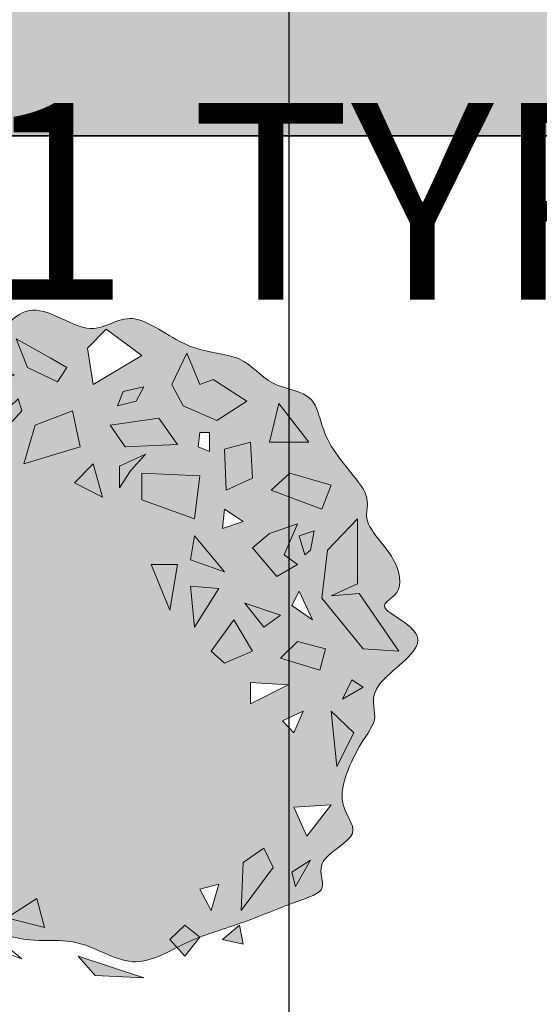
# Model space of a CAD drawing. Units: metres. Extents: x 4298.5 to 4325.2, y 2075 to 2095.8.
# Tile 9 of 35: x 4307.1445 to 4307.6197, y 2079.0337 to 2079.9341. Entities that reach past the tile are written whole.
import ezdxf

# ---------------------------------------------------------------- set-up
doc = ezdxf.new("R2010")
doc.units = ezdxf.units.M
for name, color, linetype, lineweight in [('A-ANNO-DIMS', 2, 'Continuous', 18), ('A-WALL', 7, 'Continuous', 35), ('A-WALL-PATT', 252, 'Continuous', 13), ('L-PLNT', 94, 'Continuous', 13)]:
    doc.layers.add(name, color=color, linetype=linetype, lineweight=lineweight)
doc.layers.add('L-PLNT-PATT', color=116, linetype='Continuous', lineweight=13, true_color=0x13823e)
doc.styles.get("Standard").update_dxf_attribs({"font": 'arial.ttf'})
doc.dimstyles.get("Standard").update_dxf_attribs({"dimtxt": 0.18, "dimasz": 0.18, "dimexe": 0.18, "dimexo": 0.0625, "dimgap": 0.09, "dimtad": 0, "dimtih": 1, "dimtoh": 1, "dimdec": 4, "dimzin": 0, "dimdsep": 46, "dimtxsty": 'Standard', "dimcen": 0.09, "dimadec": 0, "dimazin": 0, "dimtfac": 1, "dimtdec": 4, "dimtofl": 0, "dimtmove": 0, "dimatfit": 3, "dimfxl": 1, "dimtolj": 1, "dimtzin": 0, "dimarcsym": 0})

# ---------------------------------------------------------------- blocks, each defined once
blk = doc.blocks.new('*U9')
for points in [[(1.237, 12.003), (0.562, 11.31), (0.764, 10.013), (2.519, 11.051)], [(-2.003, 11.656), (-1.598, 10.618), (-0.518, 10.099), (-0.181, 10.618), (-0.788, 10.964)], [(-4.432, 11.051), (-5.175, 10.359), (-3.96, 9.493), (-2.07, 10.359)], [(4.139, 11.137), (3.599, 10.013), (4.004, 9.234), (5.218, 8.715), (6.298, 9.407), (5.083, 10.186), (4.611, 10.013)], [(-5.782, 9.753), (-7.537, 9.234), (-8.009, 7.504), (-6.255, 8.455)], [(2.586, 9.926), (1.844, 9.753), (1.642, 9.234), (2.316, 9.407)], [(-1.935, 9.493), (-2.475, 8.974), (-2.273, 8.542), (-1.8, 9.061)], [(7.446, 9.32), (7.108, 7.936), (8.525, 7.936)], [(-4.837, 8.628), (-3.825, 7.85), (-4.027, 8.974)], [(0.022, 9.061), (-1.328, 8.542), (-1.733, 7.157), (0.292, 7.763)], [(1.372, 8.542), (3.126, 8.801), (3.801, 7.85), (1.912, 7.763)], [(4.611, 8.282), (4.544, 7.763), (4.949, 7.59), (4.949, 8.282)], [(6.433, 7.936), (5.488, 7.676), (5.556, 6.206), (6.501, 6.638)], [(-2.88, 7.504), (-3.15, 6.638), (-2.273, 6.725)], [(1.709, 6.292), (1.709, 7.071), (2.654, 7.504), (2.114, 6.898)], [(0.764, 7.157), (0.089, 6.465), (1.102, 5.946)], [(-5.782, 6.811), (-6.659, 6.206), (-6.524, 5.687)], [(2.519, 6.811), (2.519, 5.86), (4.409, 5.167), (4.611, 6.725)], [(7.851, 6.811), (7.176, 6.206), (8.998, 5.514), (9.335, 6.379)], [(-8.144, 6.033), (-9.359, 5.946), (-9.022, 4.735)], [(-4.567, 6.379), (-5.445, 4.475), (-3.892, 4.821)], [(5.488, 5.514), (5.421, 4.821), (6.163, 5.081)], [(8.12, 4.994), (7.108, 4.648), (6.501, 4.129), (7.378, 3.091), (8.12, 3.524), (7.648, 3.87)], [(10.28, 5.167), (9.2, 4.043), (8.998, 2.312), (10.482, 0.495), (11.765, 0.409), (10.348, 2.485), (9.335, 2.399), (10.28, 2.831)], [(8.728, 4.735), (8.188, 4.562), (8.39, 3.87), (8.593, 4.043)], [(4.409, 4.562), (4.274, 3.697), (5.488, 3.264)], [(-11.316, 1.793), (-9.831, 2.312), (-9.629, 3.437), (-10.439, 3.524)], [(3.531, 1.88), (2.856, 3.524), (3.801, 3.524)], [(-8.212, 3.091), (-8.482, 2.312), (-7.874, 2.572)], [(4.274, 2.745), (5.286, 2.658), (4.409, 1.274)], [(8.188, 2.572), (7.918, 2.053), (8.66, 1.534)], [(7.513, 1.707), (6.906, 1.274), (6.231, 2.139)], [(-6.997, 1.793), (-7.942, 1.534), (-7.469, 0.495)], [(5.826, 1.534), (5.016, 0.409), (5.488, -0.024), (6.501, 0.409)], [(-8.212, 0.409), (-9.426, 0.322), (-9.831, 0.841)], [(8.12, 0.755), (7.513, 0.149), (8.93, -0.283), (9.133, 0.495)], [(10.078, -0.629), (9.74, -1.322), (10.482, -0.889)], [(7.783, -0.803), (6.433, -1.495), (6.433, -0.716)], [(8.323, -1.754), (7.985, -2.533), (7.581, -2.1)], [(9.335, -1.754), (9.538, -3.744), (10.145, -2.533)], [(-10.034, -2.706), (-10.641, -3.312), (-10.439, -4.436), (-9.899, -3.485)], [(-8.279, -5.734), (-6.794, -5.302), (-6.997, -6.513)], [(9.335, -5.129), (8.458, -6.253), (7.985, -5.215)], [(6.096, -8.935), (6.163, -7.205), (6.906, -6.686), (7.243, -7.378)], [(8.053, -8.07), (8.593, -7.118), (7.918, -7.551)], [(5.286, -7.984), (4.611, -8.157), (5.016, -8.935)], [(-2.34, -9.195), (-1.26, -8.503), (-0.99, -9.541)], [(-4.837, -8.849), (-4.432, -9.454), (-5.985, -9.801)], [(4.071, -9.454), (3.531, -9.974), (4.071, -10.579), (4.611, -9.887)], [(6.028, -9.454), (5.421, -9.974), (6.163, -10.147)], [(-2.543, -10.06), (-3.015, -10.233), (-1.8, -10.666)], [(0.224, -10.579), (0.832, -11.272), (2.586, -11.358)]]:
    blk.add_lwpolyline(points, close=True)
blk = doc.blocks.new('*D23')
at = {"layer": 'A-ANNO-DIMS', "color": 0, "lineweight": -2, "transparency": 16777216}
for p, q in [((4308.16058, 2079.85556), (4308.16058, 2079.58806)), ((4309.16058, 2079.85556), (4309.16058, 2079.58806)), ((4308.16058, 2079.76806), (4307.98058, 2079.76806)), ((4308.98058, 2079.76806), (4308.34058, 2079.76806))]:
    blk.add_line(p, q, dxfattribs=at)
at = {"layer": 'A-ANNO-DIMS', "color": 0, "transparency": 16777216}
for points in [[(4308.34058, 2079.79806), (4308.34058, 2079.73806), (4308.16058, 2079.76806)], [(4308.98058, 2079.79806), (4308.98058, 2079.73806), (4309.16058, 2079.76806)]]:
    blk.add_solid(points, dxfattribs=at)
at = {"layer": 'Defpoints', "color": 0, "transparency": 16777216}
for p in [(4308.16058, 2079.91806), (4309.16058, 2079.91806), (4308.16058, 2079.76806)]:
    blk.add_point(p, dxfattribs=at)
at = {"layer": 'A-ANNO-DIMS', "color": 0, "transparency": 16777216, "insert": (4306.70861, 2079.76806), "char_height": 0.18, "attachment_point": 5}
blk.add_mtext('\\A1;WINDOW W1 1 TYP.', dxfattribs=at)
blk = doc.blocks.new('*D47')
at = {"layer": 'A-ANNO-DIMS', "color": 0, "lineweight": -2, "transparency": 16777216}
for p, q in [((4300.43058, 2084.49556), (4300.43058, 2074.98956)), ((4322.81058, 2084.49556), (4322.81058, 2074.98956)), ((4300.61058, 2075.16956), (4311.22515, 2075.16956)), ((4322.63058, 2075.16956), (4312.016, 2075.16956))]:
    blk.add_line(p, q, dxfattribs=at)
at = {"layer": 'A-ANNO-DIMS', "color": 0, "transparency": 16777216}
for points in [[(4300.61058, 2075.19956), (4300.61058, 2075.13956), (4300.43058, 2075.16956)], [(4322.63058, 2075.19956), (4322.63058, 2075.13956), (4322.81058, 2075.16956)]]:
    blk.add_solid(points, dxfattribs=at)
at = {"layer": 'Defpoints', "color": 0, "transparency": 16777216}
for p in [(4300.43058, 2084.55806), (4322.81058, 2084.55806), (4322.81058, 2075.16956)]:
    blk.add_point(p, dxfattribs=at)
at = {"layer": 'A-ANNO-DIMS', "color": 0, "transparency": 16777216, "insert": (4311.62058, 2075.16956), "char_height": 0.18, "attachment_point": 5}
blk.add_mtext('\\A1;22.38', dxfattribs=at)
blk = doc.blocks.new('*D54')
at = {"layer": 'A-ANNO-DIMS', "color": 0, "lineweight": -2, "transparency": 16777216}
for p, q in [((4305.59808, 2079.82806), (4299.09208, 2079.82806)), ((4299.27208, 2079.64806), (4299.27208, 2078.26002)), ((4299.27208, 2076.50806), (4299.27208, 2077.89609)), ((4309.09808, 2076.32806), (4299.09208, 2076.32806))]:
    blk.add_line(p, q, dxfattribs=at)
at = {"layer": 'A-ANNO-DIMS', "color": 0, "transparency": 16777216}
for points in [[(4299.24208, 2079.64806), (4299.30208, 2079.64806), (4299.27208, 2079.82806)], [(4299.24208, 2076.50806), (4299.30208, 2076.50806), (4299.27208, 2076.32806)]]:
    blk.add_solid(points, dxfattribs=at)
at = {"layer": 'Defpoints', "color": 0, "transparency": 16777216}
for p in [(4305.66058, 2079.82806), (4299.27208, 2076.32806), (4309.16058, 2076.32806)]:
    blk.add_point(p, dxfattribs=at)
at = {"layer": 'A-ANNO-DIMS', "color": 0, "transparency": 16777216, "insert": (4299.27208, 2078.07806), "char_height": 0.18, "attachment_point": 5}
blk.add_mtext('\\A1;3.5', dxfattribs=at)
blk = doc.blocks.new('*D59')
at = {"layer": 'A-ANNO-DIMS', "color": 0, "lineweight": -2, "transparency": 16777216}
for p, q in [((4305.89058, 2079.99556), (4305.89058, 2074.98956)), ((4307.39058, 2079.99556), (4307.39058, 2074.98956)), ((4306.07058, 2075.16956), (4306.39452, 2075.16956)), ((4307.21058, 2075.16956), (4306.88663, 2075.16956))]:
    blk.add_line(p, q, dxfattribs=at)
at = {"layer": 'A-ANNO-DIMS', "color": 0, "transparency": 16777216}
for points in [[(4306.07058, 2075.19956), (4306.07058, 2075.13956), (4305.89058, 2075.16956)], [(4307.21058, 2075.19956), (4307.21058, 2075.13956), (4307.39058, 2075.16956)]]:
    blk.add_solid(points, dxfattribs=at)
at = {"layer": 'Defpoints', "color": 0, "transparency": 16777216}
for p in [(4305.89058, 2080.05806), (4307.39058, 2080.05806), (4307.39058, 2075.16956)]:
    blk.add_point(p, dxfattribs=at)
at = {"layer": 'A-ANNO-DIMS', "color": 0, "transparency": 16777216, "insert": (4306.64058, 2075.16956), "char_height": 0.18, "attachment_point": 5}
blk.add_mtext('\\A1;1.5', dxfattribs=at)
blk = doc.blocks.new('*D78')
at = {"layer": 'A-ANNO-DIMS', "color": 0, "lineweight": -2, "transparency": 16777216}
for p, q in [((4312.4969, 2079.73934), (4312.4969, 2079.91934)), ((4312.4069, 2079.82934), (4312.5869, 2079.82934)), ((4305.38467, 2076.78063), (4307.88631, 2077.85298)), ((4305.20467, 2076.78063), (4305.38467, 2076.78063))]:
    blk.add_line(p, q, dxfattribs=at)
at = {"layer": 'A-ANNO-DIMS', "color": 0, "transparency": 16777216}
blk.add_solid([(4307.87449, 2077.88055), (4307.89813, 2077.8254), (4308.05176, 2077.92389)], dxfattribs=at)
at = {"layer": 'Defpoints', "color": 0, "transparency": 16777216}
for p in [(4312.4969, 2079.82934), (4308.05176, 2077.92389)]:
    blk.add_point(p, dxfattribs=at)
at = {"layer": 'A-ANNO-DIMS', "color": 0, "transparency": 16777216, "insert": (4304.52998, 2076.78063), "char_height": 0.18, "attachment_point": 5}
blk.add_mtext('\\A1;2X R4.836', dxfattribs=at)

msp = doc.modelspace()

# ---------------------------------------------------------------- hatches: boundary and pattern name
at = {"layer": 'A-WALL-PATT'}
h = msp.add_hatch(color=256, dxfattribs=at)
h.dxf.hatch_style = 1
h.paths.add_polyline_path([(4308.76058, 2094.47806), (4308.16058, 2094.47806), (4307.46058, 2094.47806), (4307.46058, 2094.24806), (4308.27058, 2094.24806), (4308.27058, 2094.12806), (4308.39058, 2094.12806), (4308.39058, 2094.24806), (4308.76058, 2094.24806)])
h.paths.add_polyline_path([(4310.12058, 2094.47806), (4309.52058, 2094.47806), (4309.52058, 2094.24806), (4309.89058, 2094.24806), (4309.89058, 2092.24806), (4308.39058, 2092.24806), (4308.39058, 2093.42806), (4308.27058, 2093.42806), (4308.27058, 2092.01806), (4309.89058, 2092.01806), (4309.89058, 2087.01806), (4309.77058, 2087.01806), (4309.77058, 2086.78806), (4309.89058, 2086.78806), (4311.94058, 2086.78806), (4311.94058, 2087.01806), (4310.12058, 2087.01806), (4310.12058, 2089.01806), (4310.24058, 2089.01806), (4310.24058, 2089.13806), (4310.12058, 2089.13806), (4310.12058, 2092.01806), (4310.30785, 2092.01806), (4310.30785, 2092.24806), (4310.12058, 2092.24806)])
h.paths.add_polyline_path([(4311.74058, 2092.24806), (4311.06785, 2092.24806), (4311.06785, 2092.01806), (4311.74058, 2092.01806)], flags=17)
h.paths.add_polyline_path([(4313.17331, 2092.24806), (4312.50058, 2092.24806), (4312.50058, 2092.01806), (4313.17331, 2092.01806)])
h.paths.add_polyline_path([(4314.53785, 2092.24806), (4314.12058, 2092.24806), (4313.93331, 2092.24806), (4313.93331, 2092.01806), (4314.12058, 2092.01806), (4314.12058, 2087.01806), (4314.00058, 2087.01806), (4314.00058, 2086.78806), (4314.12058, 2086.78806), (4315.57179, 2086.78806), (4315.57179, 2087.01806), (4314.35058, 2087.01806), (4314.35058, 2092.01806), (4314.53785, 2092.01806)])
h.paths.add_polyline_path([(4315.97058, 2092.24806), (4315.29785, 2092.24806), (4315.29785, 2092.01806), (4315.97058, 2092.01806)])
h.paths.add_polyline_path([(4317.40331, 2092.24806), (4316.73058, 2092.24806), (4316.73058, 2092.01806), (4317.40331, 2092.01806)])
h.paths.add_polyline_path([(4318.95058, 2092.24806), (4318.35058, 2092.24806), (4318.16331, 2092.24806), (4318.16331, 2092.01806), (4318.35058, 2092.01806), (4318.35058, 2091.89806), (4318.58058, 2091.89806), (4318.58058, 2092.01806), (4318.95058, 2092.01806)])
h.paths.add_polyline_path([(4321.01058, 2092.24806), (4319.71058, 2092.24806), (4319.71058, 2092.01806), (4320.08058, 2092.01806), (4320.08058, 2090.01806), (4318.58058, 2090.01806), (4318.58058, 2091.19806), (4318.35058, 2091.19806), (4318.35058, 2090.01806), (4318.35058, 2087.01806), (4318.23058, 2087.01806), (4318.23058, 2086.78806), (4318.35058, 2086.78806), (4318.35058, 2086.30806), (4318.58058, 2086.30806), (4318.58058, 2089.78806), (4321.78058, 2089.78806), (4321.78058, 2090.01806), (4320.20058, 2090.01806), (4320.20058, 2092.01806), (4321.01058, 2092.01806)])
h.paths.add_polyline_path([(4322.81058, 2092.24806), (4321.77058, 2092.24806), (4321.77058, 2092.01806), (4322.58058, 2092.01806), (4322.58058, 2091.28306), (4322.81058, 2091.28306)])
h.paths.add_polyline_path([(4322.81058, 2090.52306), (4322.58058, 2090.52306), (4322.58058, 2089.78806), (4322.58058, 2089.52545), (4322.81058, 2089.52545), (4322.81058, 2090.01806)])
h.paths.add_polyline_path([(4322.81058, 2088.76545), (4322.58058, 2088.76545), (4322.58058, 2087.66806), (4322.81058, 2087.66806)])
h.paths.add_polyline_path([(4322.81058, 2086.90806), (4322.58058, 2086.90806), (4322.58058, 2085.81066), (4322.81058, 2085.81066)])
h.paths.add_polyline_path([(4322.81058, 2085.05066), (4322.58058, 2085.05066), (4322.58058, 2084.78806), (4318.58058, 2084.78806), (4318.58058, 2085.05806), (4318.58058, 2085.40806), (4318.35058, 2085.40806), (4318.35058, 2084.55806), (4318.35058, 2080.85806), (4318.47058, 2080.85806), (4318.47058, 2082.32806), (4319.26058, 2082.32806), (4319.26058, 2082.55806), (4318.58058, 2082.55806), (4318.58058, 2084.55806), (4320.08058, 2084.55806), (4320.08058, 2083.93806), (4320.31058, 2083.93806), (4320.31058, 2084.55806), (4322.81058, 2084.55806)])
h.paths.add_polyline_path([(4320.31058, 2083.17806), (4320.08058, 2083.17806), (4320.08058, 2082.55806), (4319.96058, 2082.55806), (4319.96058, 2082.32806), (4320.08058, 2082.32806), (4320.08058, 2081.57306), (4320.31058, 2081.57306)], flags=17)
h.paths.add_polyline_path([(4320.31058, 2080.81306), (4320.08058, 2080.81306), (4320.08058, 2080.05806), (4318.42861, 2080.05806), (4318.42861, 2079.82806), (4320.31058, 2079.82806)])
h.paths.add_polyline_path([(4317.35058, 2085.28806), (4316.57179, 2085.28806), (4316.57179, 2085.05806), (4317.35058, 2085.05806)])
h.paths.add_polyline_path([(4315.57179, 2085.28806), (4314.84342, 2085.28806), (4314.84342, 2085.05806), (4315.57179, 2085.05806)])
h.paths.add_polyline_path([(4313.84342, 2085.28806), (4312.94058, 2085.28806), (4312.94058, 2085.05806), (4313.84342, 2085.05806)])
h.paths.add_polyline_path([(4311.94058, 2085.28806), (4311.44058, 2085.28806), (4311.44058, 2085.05806), (4311.94058, 2085.05806)])
h.paths.add_polyline_path([(4317.33058, 2087.01806), (4316.57179, 2087.01806), (4316.57179, 2086.78806), (4317.33058, 2086.78806)])
h.paths.add_polyline_path([(4313.10058, 2089.13806), (4311.14058, 2089.13806), (4311.14058, 2089.01806), (4312.98058, 2089.01806), (4312.98058, 2087.01806), (4312.94058, 2087.01806), (4312.94058, 2086.78806), (4313.10058, 2086.78806), (4313.10058, 2087.01806)])
h.paths.add_polyline_path([(4307.55152, 2087.01806), (4305.89058, 2087.01806), (4305.89058, 2092.24806), (4305.89058, 2094.24806), (4306.70058, 2094.24806), (4306.70058, 2094.47806), (4305.66058, 2094.47806), (4305.66058, 2092.24806), (4305.29058, 2092.24806), (4305.29058, 2092.01806), (4305.66058, 2092.01806), (4305.66058, 2090.01806), (4304.16058, 2090.01806), (4304.16058, 2091.19806), (4304.04058, 2091.19806), (4304.04058, 2089.90806), (4301.56058, 2089.90806), (4301.56058, 2089.78806), (4304.04058, 2089.78806), (4305.66058, 2089.78806), (4305.66058, 2086.63806), (4305.89058, 2086.63806), (4305.89058, 2086.78806), (4307.55152, 2086.78806)])
h.paths.add_polyline_path([(4307.55152, 2085.28806), (4305.89058, 2085.28806), (4305.89058, 2085.43806), (4305.66058, 2085.43806), (4305.66058, 2084.78806), (4305.29058, 2084.78806), (4305.29058, 2084.55806), (4305.66058, 2084.55806), (4305.66058, 2084.02001), (4305.89058, 2084.02001), (4305.89058, 2084.55806), (4305.89058, 2085.05806), (4307.55152, 2085.05806)])
h.paths.add_polyline_path([(4310.24058, 2085.28806), (4308.55152, 2085.28806), (4308.55152, 2085.05806), (4310.24058, 2085.05806)])
h.paths.add_polyline_path([(4317.42861, 2080.05806), (4316.57179, 2080.05806), (4316.57179, 2079.82806), (4317.42861, 2079.82806)])
h.paths.add_polyline_path([(4315.57179, 2080.05806), (4314.84342, 2080.05806), (4314.84342, 2079.82806), (4315.57179, 2079.82806)])
h.paths.add_polyline_path([(4313.84342, 2080.05806), (4312.94058, 2080.05806), (4312.94058, 2079.82806), (4313.84342, 2079.82806)])
h.paths.add_polyline_path([(4311.94058, 2080.05806), (4311.44058, 2080.05806), (4311.44058, 2079.82806), (4311.94058, 2079.82806)])
h.paths.add_polyline_path([(4310.24058, 2080.05806), (4310.12058, 2080.05806), (4310.12058, 2084.03806), (4309.89058, 2084.03806), (4309.89058, 2080.05806), (4309.16058, 2080.05806), (4309.16058, 2079.82806), (4310.24058, 2079.82806)])
h.paths.add_polyline_path([(4308.16058, 2080.05806), (4307.51058, 2080.05806), (4307.51058, 2080.17806), (4307.39058, 2080.17806), (4307.39058, 2080.05806), (4305.89058, 2080.05806), (4305.89058, 2080.56697), (4305.66058, 2080.56697), (4305.66058, 2079.82806), (4308.16058, 2079.82806)])
h.paths.add_polyline_path([(4307.51058, 2081.93806), (4309.09058, 2081.93806), (4309.09058, 2082.05806), (4305.89058, 2082.05806), (4305.89058, 2083.26001), (4305.66058, 2083.26001), (4305.66058, 2081.32697), (4305.89058, 2081.32697), (4305.89058, 2081.93806), (4307.39058, 2081.93806), (4307.39058, 2080.87806), (4307.51058, 2080.87806)])
h.paths.add_polyline_path([(4304.53058, 2084.78806), (4302.73058, 2084.78806), (4302.73058, 2084.55806), (4304.53058, 2084.55806)])
h.paths.add_polyline_path([(4301.97058, 2084.78806), (4300.66058, 2084.78806), (4300.66058, 2085.02492), (4300.43058, 2085.02492), (4300.43058, 2084.55806), (4301.97058, 2084.55806)])
h.paths.add_polyline_path([(4300.66058, 2086.88429), (4300.43058, 2086.88429), (4300.43058, 2085.78492), (4300.66058, 2085.78492)])
h.paths.add_polyline_path([(4300.66058, 2089.16182), (4300.43058, 2089.16182), (4300.43058, 2087.64429), (4300.66058, 2087.64429)])
h.paths.add_polyline_path([(4300.66058, 2091.02119), (4300.43058, 2091.02119), (4300.43058, 2089.92182), (4300.66058, 2089.92182)])
h.paths.add_polyline_path([(4300.66058, 2092.01806), (4301.97058, 2092.01806), (4301.97058, 2092.24806), (4300.43058, 2092.24806), (4300.43058, 2091.78119), (4300.66058, 2091.78119)])
h.paths.add_polyline_path([(4304.53058, 2092.24806), (4302.73058, 2092.24806), (4302.73058, 2092.01806), (4304.04058, 2092.01806), (4304.04058, 2091.89806), (4304.16058, 2091.89806), (4304.16058, 2092.01806), (4304.53058, 2092.01806)], flags=17)
at = {"layer": 'L-PLNT-PATT'}
h = msp.add_hatch(color=256, dxfattribs=at)
h.dxf.hatch_style = 1
edge = h.paths.add_edge_path()
edge.add_spline(control_points=[(4307.28832, 2079.08578), (4307.29089, 2079.08709), (4307.30952, 2079.09641), (4307.34532, 2079.10618), (4307.39985, 2079.12944), (4307.4292, 2079.13707), (4307.41047, 2079.16551), (4307.46306, 2079.18971), (4307.42932, 2079.21603), (4307.45635, 2079.27577), (4307.47508, 2079.29524), (4307.45845, 2079.32373), (4307.53267, 2079.3686), (4307.46273, 2079.39817), (4307.49542, 2079.40581), (4307.49143, 2079.44094), (4307.45332, 2079.47755), (4307.47191, 2079.4969), (4307.41885, 2079.54789), (4307.41885, 2079.59392), (4307.37099, 2079.5973), (4307.35056, 2079.62919), (4307.29734, 2079.62919), (4307.24502, 2079.67454), (4307.21022, 2079.63742), (4307.14954, 2079.68828), (4307.10964, 2079.61822), (4307.06508, 2079.64819), (4307.05073, 2079.60881), (4307.01044, 2079.5858), (4307.00408, 2079.58183)], knot_values=[0.818571, 0.818571, 0.818571, 0.818571, 0.97924, 1.97924, 2.97924, 3.97924, 4.97924, 5.97924, 6.97924, 7.97924, 8.97924, 9.97924, 10.97924, 11.97924, 12.97924, 13.97924, 14.97924, 15.97924, 16.97924, 17.97924, 18.97924, 19.97924, 20.97924, 21.97924, 22.97924, 23.97924, 24.97924, 25.97924, 26.97924, 27.16067, 27.16067, 27.16067, 27.16067], degree=3, periodic=0)
edge.add_line((4307.00408, 2079.58183), (4307.04535, 2079.59404))
edge.add_line((4307.04535, 2079.59404), (4307.03333, 2079.56107))
edge.add_line((4307.03333, 2079.56107), (4306.98878, 2079.53691))
edge.add_line((4306.98878, 2079.53691), (4307.0004, 2079.5795))
edge.add_spline(control_points=[(4307.0004, 2079.5795), (4306.97776, 2079.56484), (4306.95447, 2079.5439), (4306.95719, 2079.49949)], knot_values=[0.141368, 0.141368, 0.141368, 0.141368, 0.783694, 0.783694, 0.783694, 0.783694], degree=3, periodic=0)
edge.add_spline(control_points=[(4306.95719, 2079.49949), (4306.96117, 2079.49923), (4306.9654, 2079.49889), (4306.96992, 2079.49844)], knot_values=[40.901028, 40.901028, 40.901028, 40.901028, 41, 41, 41, 41], degree=3, periodic=0)
edge.add_line((4306.96992, 2079.49844), (4306.98535, 2079.49955))
edge.add_line((4306.98535, 2079.49955), (4306.96305, 2079.46658))
edge.add_line((4306.96305, 2079.46658), (4306.95449, 2079.49734))
edge.add_line((4306.95449, 2079.49734), (4306.95732, 2079.49754))
edge.add_spline(control_points=[(4306.95733, 2079.49754), (4306.95728, 2079.4982), (4306.95723, 2079.49885), (4306.95719, 2079.49949)], knot_values=[0.13204, 0.13204, 0.13204, 0.13204, 0.141368, 0.141368, 0.141368, 0.141368], degree=3, periodic=0)
edge.add_spline(control_points=[(4306.95719, 2079.49949), (4306.92097, 2079.50184), (4306.88937, 2079.49199), (4306.83734, 2079.53397), (4306.90442, 2079.43142), (4306.90674, 2079.40456), (4306.90744, 2079.39708)], knot_values=[37.439141, 37.439141, 37.439141, 37.439141, 38.340169, 39.340169, 40.340169, 40.901028, 40.901028, 40.901028, 40.901028], degree=3, periodic=0)
edge.add_line((4306.90744, 2079.39708), (4306.92706, 2079.43582))
edge.add_line((4306.92706, 2079.43582), (4306.94764, 2079.43361))
edge.add_line((4306.94764, 2079.43361), (4306.9425, 2079.40504))
edge.add_line((4306.9425, 2079.40504), (4306.90786, 2079.39293))
edge.add_spline(control_points=[(4306.90786, 2079.39293), (4306.90835, 2079.38899), (4306.91143, 2079.37544), (4306.95279, 2079.35449), (4306.93133, 2079.25721), (4306.96358, 2079.23836), (4307.0298, 2079.23836), (4307.05256, 2079.18462), (4307.05606, 2079.14915), (4307.13706, 2079.08309), (4307.19535, 2079.09986), (4307.24573, 2079.06298), (4307.27487, 2079.07895), (4307.28832, 2079.08578)], knot_values=[27.16067, 27.16067, 27.16067, 27.16067, 27.490087, 28.490087, 29.490087, 30.490087, 31.490087, 32.490087, 33.490087, 34.490087, 35.490087, 36.490087, 37.329418, 37.329418, 37.329418, 37.329418], degree=3, periodic=0)
edge.add_line((4307.28832, 2079.08578), (4307.2819, 2079.09297))
edge.add_line((4307.2819, 2079.09297), (4307.29562, 2079.10618))
edge.add_line((4307.29562, 2079.10618), (4307.30934, 2079.09517))
h.paths.add_polyline_path([(4307.26475, 2079.43582), (4307.28876, 2079.43582), (4307.2819, 2079.39406)], flags=16)
h.paths.add_polyline_path([(4307.30077, 2079.41603), (4307.32648, 2079.41382), (4307.3042, 2079.37867)], flags=16)
h.paths.add_polyline_path([(4307.09335, 2079.46876), (4307.05391, 2079.45998), (4307.07621, 2079.50834)], flags=16)
h.paths.add_polyline_path([(4307.2202, 2079.49734), (4307.19447, 2079.51052), (4307.21162, 2079.5281)], flags=16)
h.paths.add_polyline_path([(4307.30077, 2079.44022), (4307.3042, 2079.46219), (4307.33161, 2079.42922)], flags=16)
h.paths.add_polyline_path([(4307.31962, 2079.3567), (4307.34019, 2079.38527), (4307.35734, 2079.3567), (4307.33161, 2079.3457)], flags=16)
h.paths.add_polyline_path([(4307.25619, 2079.49516), (4307.25619, 2079.51931), (4307.30933, 2079.51713), (4307.3042, 2079.47755)], flags=16)
h.paths.add_polyline_path([(4307.23562, 2079.50613), (4307.23562, 2079.52591), (4307.25962, 2079.53691), (4307.24591, 2079.52152)], flags=16)
h.paths.add_polyline_path([(4307.13448, 2079.51713), (4307.1122, 2079.51492), (4307.11906, 2079.53691)], flags=16)
h.paths.add_polyline_path([(4307.14819, 2079.5281), (4307.15848, 2079.56328), (4307.19277, 2079.57646), (4307.19963, 2079.54349)], flags=16)
h.paths.add_polyline_path([(4307.01449, 2079.39185), (4307.0025, 2079.35888), (4306.99048, 2079.38527)], flags=16)
h.paths.add_polyline_path([(4307.35048, 2079.40064), (4307.38304, 2079.38967), (4307.36762, 2079.37867)], flags=16)
h.paths.add_polyline_path([(4307.32991, 2079.46876), (4307.33161, 2079.48637), (4307.34875, 2079.47537)], flags=16)
h.paths.add_polyline_path([(4307.24078, 2079.54349), (4307.22706, 2079.56328), (4307.27161, 2079.56986), (4307.28876, 2079.5457)], flags=16)
h.paths.add_polyline_path([(4307.35561, 2079.32812), (4307.3899, 2079.32592), (4307.35561, 2079.30834)], flags=16)
h.paths.add_polyline_path([(4306.99221, 2079.41164), (4306.97677, 2079.40504), (4306.98363, 2079.42482)], flags=16)
h.paths.add_polyline_path([(4307.09506, 2079.5457), (4307.06935, 2079.56546), (4307.08993, 2079.57425)], flags=16)
h.paths.add_polyline_path([(4307.0265, 2079.49076), (4307.02307, 2079.50394), (4307.04535, 2079.51931)], flags=16)
h.paths.add_polyline_path([(4307.13448, 2079.56328), (4307.12935, 2079.57425), (4307.14306, 2079.58743), (4307.14649, 2079.57646)], flags=16)
h.paths.add_polyline_path([(4307.35734, 2079.45119), (4307.37275, 2079.46437), (4307.39846, 2079.47316), (4307.38647, 2079.44461), (4307.39846, 2079.43582), (4307.37961, 2079.42482)], flags=16)
h.paths.add_polyline_path([(4306.98363, 2079.3567), (4306.95279, 2079.35449), (4306.9425, 2079.36767)], flags=16)
h.paths.add_polyline_path([(4307.33333, 2079.50394), (4307.33161, 2079.54128), (4307.35561, 2079.54789), (4307.35734, 2079.51492)], flags=16)
h.paths.add_polyline_path([(4307.38304, 2079.3501), (4307.39846, 2079.36549), (4307.42419, 2079.35888), (4307.41903, 2079.33912)], flags=16)
h.paths.add_polyline_path([(4307.30763, 2079.54349), (4307.30933, 2079.55667), (4307.31792, 2079.55667), (4307.31792, 2079.5391)], flags=16)
h.paths.add_polyline_path([(4307.23392, 2079.58085), (4307.23905, 2079.59404), (4307.2579, 2079.59843), (4307.25104, 2079.58525)], flags=16)
h.paths.add_polyline_path([(4307.39333, 2079.39846), (4307.40019, 2079.41164), (4307.41218, 2079.38527)], flags=16)
h.paths.add_polyline_path([(4307.38477, 2079.29297), (4307.40362, 2079.30176), (4307.39503, 2079.28197)], flags=16)
h.paths.add_polyline_path([(4307.17905, 2079.60283), (4307.15162, 2079.61601), (4307.14134, 2079.64237), (4307.1722, 2079.6248), (4307.18761, 2079.61601)], flags=16)
h.paths.add_polyline_path([(4307.21162, 2079.60064), (4307.20649, 2079.63359), (4307.22363, 2079.65119), (4307.25619, 2079.62701)], flags=16)
h.paths.add_polyline_path([(4307.09163, 2079.58743), (4307.06077, 2079.60943), (4307.07964, 2079.62701), (4307.13963, 2079.60943)], flags=16)
h.paths.add_polyline_path([(4307.37448, 2079.50394), (4307.39163, 2079.51931), (4307.42932, 2079.50834), (4307.42076, 2079.48637)], flags=16)
h.paths.add_polyline_path([(4307.29391, 2079.58085), (4307.28363, 2079.60064), (4307.29734, 2079.62919), (4307.30933, 2079.60064), (4307.32132, 2079.60504), (4307.35218, 2079.58525), (4307.32475, 2079.56767)], flags=16)
h.paths.add_polyline_path([(4307.40532, 2079.44461), (4307.40019, 2079.46219), (4307.4139, 2079.46658), (4307.41047, 2079.449)], flags=16)
h.paths.add_polyline_path([(4307.42076, 2079.40504), (4307.42589, 2079.449), (4307.45332, 2079.47755), (4307.45332, 2079.41822), (4307.42932, 2079.40725), (4307.45505, 2079.40943), (4307.49104, 2079.3567), (4307.45845, 2079.35888)], flags=16)
h.paths.add_polyline_path([(4307.16021, 2079.13034), (4307.16707, 2079.10397), (4307.13278, 2079.11276)], flags=16)
h.paths.add_polyline_path([(4307.37275, 2079.54789), (4307.38134, 2079.58304), (4307.40875, 2079.54789)], flags=16)
h.paths.add_polyline_path([(4307.42932, 2079.30176), (4307.44989, 2079.28197), (4307.43448, 2079.25121)], flags=16)
h.paths.add_polyline_path([(4307.43961, 2079.31273), (4307.44819, 2079.33033), (4307.45845, 2079.32373)], flags=16)
h.paths.add_polyline_path([(4307.30933, 2079.13912), (4307.32648, 2079.14352), (4307.31962, 2079.11936)], flags=16)
h.paths.add_polyline_path([(4307.39503, 2079.21385), (4307.42932, 2079.21603), (4307.40704, 2079.18749)], flags=16)
h.paths.add_polyline_path([(4307.34875, 2079.1633), (4307.36762, 2079.17649), (4307.37618, 2079.15891), (4307.34705, 2079.11936)], flags=16)
h.paths.add_polyline_path([(4307.39333, 2079.15452), (4307.41047, 2079.16551), (4307.39676, 2079.14133)], flags=16)
h = msp.add_hatch(color=256, dxfattribs=at)
h.dxf.hatch_style = 1
h.paths.add_polyline_path([(4307.3042, 2079.47755), (4307.30933, 2079.51713), (4307.25619, 2079.51931), (4307.25619, 2079.49516)])
h.paths.add_polyline_path([(4307.35048, 2079.40064), (4307.36762, 2079.37867), (4307.38304, 2079.38967)])
h.paths.add_polyline_path([(4307.33161, 2079.54128), (4307.33333, 2079.50394), (4307.35734, 2079.51492), (4307.35561, 2079.54789)])
h.paths.add_polyline_path([(4307.35218, 2079.58525), (4307.32132, 2079.60504), (4307.30933, 2079.60064), (4307.29734, 2079.62919), (4307.28363, 2079.60064), (4307.29391, 2079.58085), (4307.32475, 2079.56767)])
h.paths.add_polyline_path([(4307.1979, 2079.0776), (4307.21334, 2079.06), (4307.2579, 2079.05782)])
h.paths.add_polyline_path([(4307.17905, 2079.60283), (4307.18761, 2079.61601), (4307.1722, 2079.6248), (4307.14134, 2079.64237), (4307.15162, 2079.61601)])
h.paths.add_polyline_path([(4307.07964, 2079.62701), (4307.06077, 2079.60943), (4307.09163, 2079.58743), (4307.13963, 2079.60943)])
h.paths.add_polyline_path([(4307.15848, 2079.56328), (4307.14819, 2079.5281), (4307.19963, 2079.54349), (4307.19277, 2079.57646)])
h.paths.add_polyline_path([(4307.14649, 2079.57646), (4307.14306, 2079.58743), (4307.12935, 2079.57425), (4307.13448, 2079.56328)])
h.paths.add_polyline_path([(4307.11906, 2079.53691), (4307.1122, 2079.51492), (4307.13448, 2079.51713)])
h.paths.add_polyline_path([(4307.09506, 2079.5457), (4307.08993, 2079.57425), (4307.06935, 2079.56546)])
h.paths.add_polyline_path([(4307.00077, 2079.58085), (4306.98878, 2079.53691), (4307.03333, 2079.56107), (4307.04535, 2079.59404)])
h.paths.add_polyline_path([(4307.04535, 2079.51931), (4307.02307, 2079.50394), (4307.0265, 2079.49076)])
h.paths.add_polyline_path([(4306.95449, 2079.49734), (4306.96305, 2079.46658), (4306.98535, 2079.49955)])
h.paths.add_polyline_path([(4306.90479, 2079.39185), (4306.9425, 2079.40504), (4306.94764, 2079.43361), (4306.92706, 2079.43582)])
h.paths.add_polyline_path([(4307.01449, 2079.39185), (4306.99048, 2079.38527), (4307.0025, 2079.35888)])
h.paths.add_polyline_path([(4306.94078, 2079.25779), (4306.93735, 2079.27758), (4306.92193, 2079.26219), (4306.92706, 2079.23364)])
h.paths.add_polyline_path([(4307.01964, 2079.21164), (4306.98193, 2079.20067), (4307.01449, 2079.18088)])
h.paths.add_polyline_path([(4307.04019, 2079.09737), (4307.07964, 2079.10618), (4307.06935, 2079.12155)])
h.paths.add_polyline_path([(4307.16021, 2079.13034), (4307.13278, 2079.11276), (4307.16707, 2079.10397)])
h.paths.add_polyline_path([(4307.29562, 2079.10618), (4307.2819, 2079.09297), (4307.29562, 2079.0776), (4307.30933, 2079.09518)])
h.paths.add_polyline_path([(4307.37618, 2079.15891), (4307.36762, 2079.17649), (4307.34875, 2079.1633), (4307.34705, 2079.11936)])
h.paths.add_polyline_path([(4307.34532, 2079.10618), (4307.32991, 2079.09297), (4307.34875, 2079.08858)])
h.paths.add_polyline_path([(4307.39333, 2079.15452), (4307.39676, 2079.14133), (4307.41047, 2079.16551)])
h.paths.add_polyline_path([(4307.43448, 2079.25121), (4307.44989, 2079.28197), (4307.42932, 2079.30176)])
h.paths.add_polyline_path([(4307.31962, 2079.3567), (4307.33161, 2079.3457), (4307.35734, 2079.3567), (4307.34019, 2079.38527)])
h.paths.add_polyline_path([(4307.45845, 2079.35888), (4307.49104, 2079.3567), (4307.45505, 2079.40943), (4307.42932, 2079.40725), (4307.45332, 2079.41822), (4307.45332, 2079.47755), (4307.42589, 2079.449), (4307.42076, 2079.40504)])
h.paths.add_polyline_path([(4307.39846, 2079.36549), (4307.38304, 2079.3501), (4307.41903, 2079.33912), (4307.42419, 2079.35888)])
h.paths.add_polyline_path([(4307.45845, 2079.32373), (4307.44819, 2079.33033), (4307.43961, 2079.31273)])
h.paths.add_polyline_path([(4307.39846, 2079.47316), (4307.37275, 2079.46437), (4307.35734, 2079.45119), (4307.37961, 2079.42482), (4307.39846, 2079.43582), (4307.38647, 2079.44461)])
h.paths.add_polyline_path([(4307.40019, 2079.46219), (4307.40532, 2079.44461), (4307.41047, 2079.449), (4307.4139, 2079.46658)])
h.paths.add_polyline_path([(4307.42076, 2079.48637), (4307.42932, 2079.50834), (4307.39163, 2079.51931), (4307.37448, 2079.50394)])
h.paths.add_polyline_path([(4307.33161, 2079.42922), (4307.3042, 2079.46219), (4307.30077, 2079.44022)])
h.paths.add_polyline_path([(4307.28876, 2079.43582), (4307.26475, 2079.43582), (4307.2819, 2079.39406)])
h.paths.add_polyline_path([(4307.32648, 2079.41382), (4307.30077, 2079.41603), (4307.3042, 2079.37867)])
h.paths.add_polyline_path([(4307.28876, 2079.5457), (4307.27161, 2079.56986), (4307.22706, 2079.56328), (4307.24078, 2079.54349)])
h.paths.add_polyline_path([(4307.24591, 2079.52152), (4307.25962, 2079.53691), (4307.23562, 2079.52591), (4307.23562, 2079.50613)])
h.paths.add_polyline_path([(4307.21162, 2079.5281), (4307.19447, 2079.51052), (4307.2202, 2079.49734)])
h.paths.add_polyline_path([(4307.25104, 2079.58525), (4307.2579, 2079.59843), (4307.23905, 2079.59404), (4307.23392, 2079.58085)])
h.paths.add_polyline_path([(4307.38134, 2079.58304), (4307.37275, 2079.54789), (4307.40875, 2079.54789)])

# ---------------------------------------------------------------- linework, layer by layer
at = {"layer": 'A-WALL'}
msp.add_line((4310.24058, 2079.82806), (4305.66058, 2079.82806), dxfattribs=at)
at = {"layer": 'L-PLNT'}
msp.add_open_spline([(4306.96305, 2079.46658), (4306.93898, 2079.55309), (4307.04535, 2079.59404), (4307.06508, 2079.64819), (4307.10964, 2079.61822), (4307.14954, 2079.68828), (4307.21022, 2079.63742), (4307.24502, 2079.67454), (4307.29734, 2079.62919), (4307.35056, 2079.62919), (4307.37099, 2079.5973), (4307.41885, 2079.59392), (4307.41885, 2079.54789), (4307.47191, 2079.4969), (4307.45332, 2079.47755), (4307.49143, 2079.44094), (4307.49542, 2079.40581), (4307.46273, 2079.39817), (4307.53267, 2079.3686), (4307.45845, 2079.32373), (4307.47508, 2079.29524), (4307.45635, 2079.27577), (4307.42932, 2079.21603), (4307.46306, 2079.18971), (4307.41047, 2079.16551), (4307.4292, 2079.13707), (4307.39985, 2079.12944), (4307.34532, 2079.10618), (4307.29562, 2079.09262), (4307.24858, 2079.06089), (4307.19535, 2079.09986), (4307.13706, 2079.08309), (4307.05606, 2079.14915), (4307.05256, 2079.18462), (4307.0298, 2079.23836), (4306.96358, 2079.23836), (4306.93133, 2079.25721), (4306.95279, 2079.35449), (4306.89953, 2079.38148), (4306.91592, 2079.41384), (4306.83734, 2079.53397), (4306.89115, 2079.49056), (4306.92426, 2079.50297), (4306.96992, 2079.49844)], degree=3, dxfattribs=at)

# ---------------------------------------------------------------- block references
at = {"layer": 'L-PLNT', "xscale": 0.0254, "yscale": 0.0254, "zscale": 0.0254}
msp.add_blockref('*U9', (4307.19222, 2079.34632), dxfattribs=at)

# ---------------------------------------------------------------- dimensions: what is measured, and where the dimension line sits
at = {"layer": 'A-ANNO-DIMS'}
for base, p1, p2, override, picture, middle in [((4322.81058, 2075.16956), (4300.43058, 2084.55806), (4322.81058, 2084.55806), {"dimdec": 2, "dimlfac": 1, "dimrnd": 0, "dimzin": 0, "dimdsep": 46, "dimlunit": 2}, '*D47', (4311.62058, 2075.16956)), ((4307.39058, 2075.16956), (4305.89058, 2080.05806), (4307.39058, 2080.05806), {"dimdec": 1, "dimlfac": 1, "dimrnd": 0, "dimzin": 0, "dimdsep": 46, "dimlunit": 2}, '*D59', (4306.64058, 2075.16956))]:
    dim = msp.add_linear_dim(base=base, p1=p1, p2=p2, dimstyle='Standard', override=override, dxfattribs=at)
    dim.commit()
    dim.dimension.update_dxf_attribs({"geometry": picture, "text_midpoint": middle})
dim = msp.add_linear_dim(base=(4308.16058, 2079.76806), p1=(4309.16058, 2079.91806), p2=(4308.16058, 2079.91806), angle=180, text='WINDOW W1 <> TYP.', dimstyle='Standard', override={"dimdec": 0, "dimlfac": 1, "dimrnd": 0, "dimzin": 0, "dimdsep": 46, "dimlunit": 2}, dxfattribs=at)
dim.commit()
dim.dimension.update_dxf_attribs({"geometry": '*D23', "text_midpoint": (4306.70861, 2079.76806)})
dim = msp.add_radius_dim(center=(4312.4969, 2079.82934), mpoint=(4308.05176, 2077.92389), text='2X <>', dimstyle='Standard', override={"dimdec": 3, "dimlfac": 1, "dimrnd": 0, "dimzin": 0, "dimdsep": 46, "dimlunit": 2}, dxfattribs=at)
dim.commit()
dim.dimension.update_dxf_attribs({"geometry": '*D78', "text_midpoint": (4304.52998, 2076.78063), "dimtype": 164})
dim = msp.add_linear_dim(base=(4299.27208, 2076.32806), p1=(4305.66058, 2079.82806), p2=(4309.16058, 2076.32806), angle=90, dimstyle='Standard', override={"dimdec": 1, "dimlfac": 1, "dimrnd": 0, "dimzin": 0, "dimdsep": 46, "dimlunit": 2}, dxfattribs=at)
dim.commit()
dim.dimension.update_dxf_attribs({"geometry": '*D54', "text_midpoint": (4299.27208, 2078.07806)})

doc.saveas('drawing.dxf')
